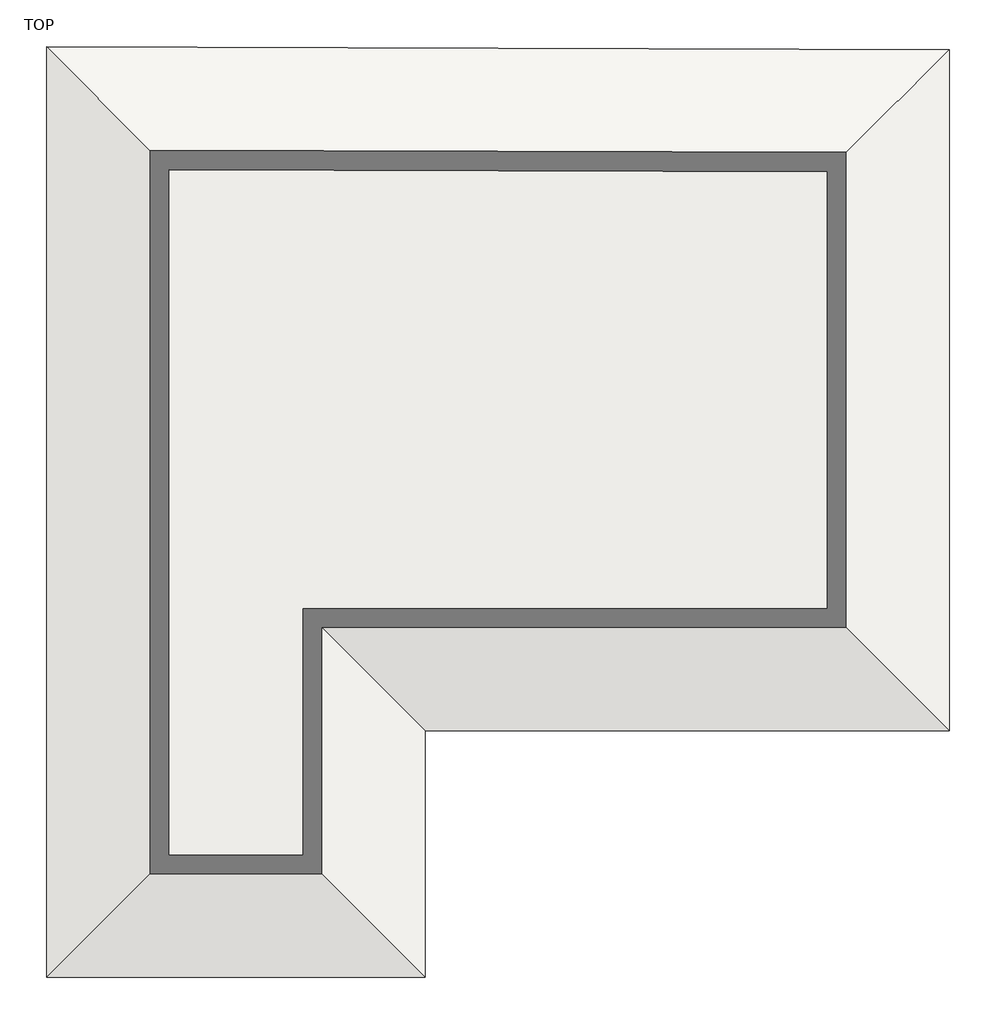
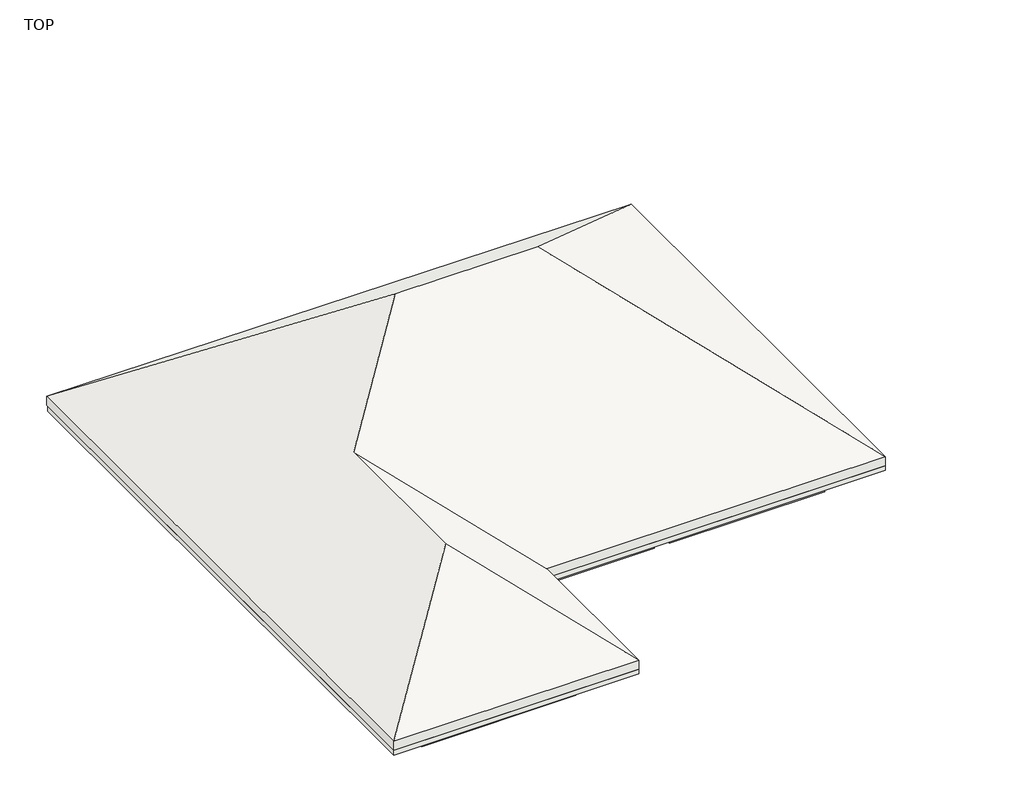
# One storey: 21 beams, 1 covering, 1 roof.
"""IFC4 building model written with IfcOpenShell, lengths in millimetres."""

from ifc_helpers import new_model, si_unit, frame, origin, place, context, project, spatial, polyline, outline, extrude, faceted_brep, element, save

model = new_model("IFC4")

# Units and contexts
model_context = context("Model", 3, world=origin())
ifc_project = project(units=[si_unit("LENGTHUNIT", "METRE", prefix="MILLI")], contexts=[model_context])

# Site, building, storey
site = spatial("IfcSite", under=ifc_project)
building = spatial("IfcBuilding", under=site)
storey = spatial("IfcBuildingStorey", under=building, Name="TOP", Elevation=6400.8)

# Beams
placement = place(None, origin())
element("IfcBeam", 1, ObjectType="Concrete-Rectangular Beam : 12 x 24", at=placement, inside=storey, context=model_context, shape_type="SweptSolid", body=[
    extrude(outline(polyline([(-11339.0293601, -6018.4747117), (-11643.8293601, -6018.4747117), (-11643.8293601, -2868.8747117), (-11339.0293601, -2868.8747117), (-11339.0293601, -6018.4747117)])), frame((0.0, 0.0, 5791.2), z_axis=(0.0, 0.0, 1.0), x_axis=(1.0, 0.0, 0.0)), (0.0, 0.0, 1.0), 609.6),
])
element("IfcBeam", 2, ObjectType="Concrete-Rectangular Beam : 12 x 24", at=placement, inside=storey, context=model_context, shape_type="SweptSolid", body=[
    extrude(outline(polyline([(-8251.5270642, -2564.0747117), (-8251.5270642, -2868.8747117), (-11339.0293601, -2868.8747117), (-11339.0293601, -2564.0747117), (-8251.5270642, -2564.0747117)])), frame((0.0, 0.0, 5791.2), z_axis=(0.0, 0.0, 1.0), x_axis=(1.0, 0.0, 0.0)), (0.0, 0.0, 1.0), 609.6),
])
element("IfcBeam", 3, ObjectType="Concrete-Rectangular Beam : 12 x 24", at=placement, inside=storey, context=model_context, shape_type="SweptSolid", body=[
    extrude(outline(polyline([(-4797.1270642, -2564.0747117), (-4797.1270642, -2868.8747117), (-7946.7270642, -2868.8747117), (-7946.7270642, -2564.0747117), (-4797.1270642, -2564.0747117)])), frame((0.0, 0.0, 5791.2), z_axis=(0.0, 0.0, 1.0), x_axis=(1.0, 0.0, 0.0)), (0.0, 0.0, 1.0), 609.6),
])
element("IfcBeam", 4, ObjectType="Concrete-Rectangular Beam : 12 x 24", at=placement, inside=storey, context=model_context, shape_type="SweptSolid", body=[
    extrude(outline(polyline([(-1351.9658472, -2564.0747117), (-1351.9658472, -2868.8747117), (-4492.3270642, -2868.8747117), (-4492.3270642, -2564.0747117), (-1351.9658472, -2564.0747117)])), frame((0.0, 0.0, 5791.2), z_axis=(0.0, 0.0, 1.0), x_axis=(1.0, 0.0, 0.0)), (0.0, 0.0, 1.0), 609.6),
])
element("IfcBeam", 5, ObjectType="Concrete-Rectangular Beam : 12 x 24", at=placement, inside=storey, context=model_context, shape_type="SweptSolid", body=[
    extrude(outline(polyline([(-1047.1658472, -5993.0747117), (-1351.9658472, -5993.0747117), (-1351.9658472, -2868.8747117), (-1047.1658472, -2868.8747117), (-1047.1658472, -5993.0747117)])), frame((0.0, 0.0, 5791.2), z_axis=(0.0, 0.0, 1.0), x_axis=(1.0, 0.0, 0.0)), (0.0, 0.0, 1.0), 609.6),
])
element("IfcBeam", 6, ObjectType="Concrete-Rectangular Beam : 12 x 24", at=placement, inside=storey, context=model_context, shape_type="SweptSolid", body=[
    extrude(outline(polyline([(-8251.5270642, -2868.8747117), (-7946.7270642, -2868.8747117), (-7946.7270642, -5993.0747117), (-8251.5270642, -5993.0747117), (-8251.5270642, -2868.8747117)])), frame((0.0, 0.0, 5791.2), z_axis=(0.0, 0.0, 1.0), x_axis=(1.0, 0.0, 0.0)), (0.0, 0.0, 1.0), 609.6),
    extrude(outline(polyline([(-7946.7270642, -6323.2747117), (-8251.5270642, -6323.2747117), (-8251.5270642, -6297.8747117), (-7946.7270642, -6297.8747117), (-7946.7270642, -6323.2747117)])), frame((0.0, 0.0, 5791.2), z_axis=(0.0, 0.0, 1.0), x_axis=(1.0, 0.0, 0.0)), (0.0, 0.0, 1.0), 609.6),
])
element("IfcBeam", 7, ObjectType="Concrete-Rectangular Beam : 12 x 24", at=placement, inside=storey, context=model_context, shape_type="SweptSolid", body=[
    extrude(outline(polyline([(-1047.1658472, -9984.0050402), (-1351.9658472, -9984.0050402), (-1351.9658472, -6297.8747117), (-1047.1658472, -6297.8747117), (-1047.1658472, -9984.0050402)])), frame((0.0, 0.0, 5791.2), z_axis=(0.0, 0.0, 1.0), x_axis=(1.0, 0.0, 0.0)), (0.0, 0.0, 1.0), 609.6),
])
element("IfcBeam", 8, ObjectType="Concrete-Rectangular Beam : 12 x 24", at=placement, inside=storey, context=model_context, shape_type="SweptSolid", body=[
    extrude(outline(polyline([(-4492.3270642, -10288.8050402), (-4492.3270642, -9984.0050402), (-1351.9658472, -9984.0050402), (-1351.9658472, -10288.8050402), (-4492.3270642, -10288.8050402)])), frame((0.0, 0.0, 5791.2), z_axis=(0.0, 0.0, 1.0), x_axis=(1.0, 0.0, 0.0)), (0.0, 0.0, 1.0), 609.6),
])
element("IfcBeam", 9, ObjectType="Concrete-Rectangular Beam : 12 x 24", at=placement, inside=storey, context=model_context, shape_type="Brep", body=[
    faceted_brep([(-7946.7270642, -9984.0050402, 6400.8), (-7946.7270642, -10288.8050402, 6400.8), (-7921.3270642, -10288.8050402, 6400.8), (-4797.1270642, -10288.8050402, 6400.8), (-4797.1270642, -9984.0050402, 6400.8), (-7946.7270642, -9984.0050402, 5791.2), (-4797.1270642, -9984.0050402, 5791.2), (-7946.7270642, -10288.8050402, 5791.2), (-4797.1270642, -10288.8050402, 5791.2), (-7921.3270642, -10288.8050402, 5791.2)], [[[0, 1, 2, 3, 4]], [[5, 0, 4, 6]], [[7, 5, 6, 8, 9]], [[1, 7, 9, 8, 3, 2]], [[1, 0, 5, 7]], [[3, 8, 6, 4]]]),
])
element("IfcBeam", 10, ObjectType="Concrete-Rectangular Beam : 12 x 24", at=placement, inside=storey, context=model_context, shape_type="SweptSolid", body=[
    extrude(outline(polyline([(-8251.5270642, -8902.7373391), (-7946.7270642, -8902.7373391), (-7946.7270642, -9984.0050402), (-8251.5270642, -9984.0050402), (-8251.5270642, -8902.7373391)])), frame((0.0, 0.0, 5791.2), z_axis=(0.0, 0.0, 1.0), x_axis=(1.0, 0.0, 0.0)), (0.0, 0.0, 1.0), 609.6),
])
element("IfcBeam", 11, ObjectType="Concrete-Rectangular Beam : 12 x 24", at=placement, inside=storey, context=model_context, shape_type="SweptSolid", body=[
    extrude(outline(polyline([(-7946.7270642, -8597.9373391), (-8251.5270642, -8597.9373391), (-8251.5270642, -6323.2747117), (-7946.7270642, -6323.2747117), (-7946.7270642, -8597.9373391)])), frame((0.0, 0.0, 5791.2), z_axis=(0.0, 0.0, 1.0), x_axis=(1.0, 0.0, 0.0)), (0.0, 0.0, 1.0), 609.6),
])
element("IfcBeam", 12, ObjectType="Concrete-Rectangular Beam : 12 x 24", at=placement, inside=storey, context=model_context, shape_type="SweptSolid", body=[
    extrude(outline(polyline([(-11339.0293601, -8902.7373391), (-11339.0293601, -8597.9373391), (-8251.5270642, -8597.9373391), (-8251.5270642, -8902.7373391), (-11339.0293601, -8902.7373391)])), frame((0.0, 0.0, 5791.2), z_axis=(0.0, 0.0, 1.0), x_axis=(1.0, 0.0, 0.0)), (0.0, 0.0, 1.0), 609.6),
])
element("IfcBeam", 13, ObjectType="Concrete-Rectangular Beam : 12 x 24", at=placement, inside=storey, context=model_context, shape_type="SweptSolid", body=[
    extrude(outline(polyline([(-11643.8293601, -6323.2747117), (-11339.0293601, -6323.2747117), (-11339.0293601, -8597.9373391), (-11643.8293601, -8597.9373391), (-11643.8293601, -6323.2747117)])), frame((0.0, 0.0, 5791.2), z_axis=(0.0, 0.0, 1.0), x_axis=(1.0, 0.0, 0.0)), (0.0, 0.0, 1.0), 609.6),
])
element("IfcBeam", 14, ObjectType="Concrete-Rectangular Beam : 12 x 24", at=placement, inside=storey, context=model_context, shape_type="Brep", body=[
    faceted_brep([(-8251.5270642, -6018.4747117, 6400.8), (-8251.5270642, -6297.8747117, 6400.8), (-8251.5270642, -6323.2747117, 6400.8), (-8251.5270642, -6323.2747117, 5791.2), (-8251.5270642, -6297.8747117, 5791.2), (-8251.5270642, -6018.4747117, 5791.2), (-11339.0293601, -6018.4747117, 6400.8), (-11339.0293601, -6323.2747117, 6400.8), (-11339.0293601, -6323.2747117, 5791.2), (-11339.0293601, -6018.4747117, 5791.2)], [[[0, 1, 2, 3, 4, 5]], [[2, 1, 0, 6, 7]], [[3, 2, 7, 8]], [[5, 4, 3, 8, 9]], [[0, 5, 9, 6]], [[6, 9, 8, 7]]]),
])
element("IfcBeam", 15, ObjectType="Concrete-Rectangular Beam : 12 x 24", at=placement, inside=storey, context=model_context, shape_type="SweptSolid", body=[
    extrude(outline(polyline([(-4797.1270642, -6297.8747117), (-4492.3270642, -6297.8747117), (-4492.3270642, -9984.0050402), (-4797.1270642, -9984.0050402), (-4797.1270642, -6297.8747117)])), frame((0.0, 0.0, 5791.2), z_axis=(0.0, 0.0, 1.0), x_axis=(1.0, 0.0, 0.0)), (0.0, 0.0, 1.0), 609.6),
])
element("IfcBeam", 16, ObjectType="Concrete-Rectangular Beam : 12 x 24", at=placement, inside=storey, context=model_context, shape_type="SweptSolid", body=[
    extrude(outline(polyline([(-4492.3270642, -6297.8747117), (-4492.3270642, -5993.0747117), (-1351.9658472, -5993.0747117), (-1351.9658472, -6297.8747117), (-4492.3270642, -6297.8747117)])), frame((0.0, 0.0, 5791.2), z_axis=(0.0, 0.0, 1.0), x_axis=(1.0, 0.0, 0.0)), (0.0, 0.0, 1.0), 609.6),
])
element("IfcBeam", 17, ObjectType="Concrete-Rectangular Beam : 12 x 24", at=placement, inside=storey, context=model_context, shape_type="SweptSolid", body=[
    extrude(outline(polyline([(-4797.1270642, -2868.8747117), (-4492.3270642, -2868.8747117), (-4492.3270642, -5993.0747117), (-4797.1270642, -5993.0747117), (-4797.1270642, -2868.8747117)])), frame((0.0, 0.0, 5791.2), z_axis=(0.0, 0.0, 1.0), x_axis=(1.0, 0.0, 0.0)), (0.0, 0.0, 1.0), 609.6),
])
element("IfcBeam", 18, ObjectType="Concrete-Rectangular Beam : 12 x 24", at=placement, inside=storey, context=model_context, shape_type="SweptSolid", body=[
    extrude(outline(polyline([(-4797.1270642, -5993.0747117), (-4797.1270642, -6297.8747117), (-7946.7270642, -6297.8747117), (-7946.7270642, -5993.0747117), (-4797.1270642, -5993.0747117)])), frame((0.0, 0.0, 5791.2), z_axis=(0.0, 0.0, 1.0), x_axis=(1.0, 0.0, 0.0)), (0.0, 0.0, 1.0), 609.6),
])
element("IfcBeam", 19, ObjectType="Concrete-Rectangular Beam : 12 x 24", at=placement, inside=storey, context=model_context, shape_type="SweptSolid", body=[
    extrude(outline(polyline([(-11643.8293601, -8902.7373391), (-11339.0293601, -8902.7373391), (-11339.0293601, -13183.002305), (-11643.8293601, -13183.002305), (-11643.8293601, -8902.7373391)])), frame((0.0, 0.0, 5791.2), z_axis=(0.0, 0.0, 1.0), x_axis=(1.0, 0.0, 0.0)), (0.0, 0.0, 1.0), 609.6),
])
element("IfcBeam", 20, ObjectType="Concrete-Rectangular Beam : 12 x 24", at=placement, inside=storey, context=model_context, shape_type="Brep", body=[
    faceted_brep([(-7921.3270642, -10288.8050402, 6400.8), (-7946.7270642, -10288.8050402, 6400.8), (-8226.1270642, -10288.8050402, 6400.8), (-8226.1270642, -13183.002305, 6400.8), (-7921.3270642, -13183.002305, 6400.8), (-8226.1270642, -10288.8050402, 5791.2), (-8226.1270642, -13183.002305, 5791.2), (-7946.7270642, -10288.8050402, 5791.2), (-7921.3270642, -10288.8050402, 5791.2), (-7921.3270642, -13183.002305, 5791.2)], [[[0, 1, 2, 3, 4]], [[2, 5, 6, 3]], [[5, 7, 8, 9, 6]], [[8, 0, 4, 9]], [[0, 8, 7, 5, 2, 1]], [[4, 3, 6, 9]]]),
])
element("IfcBeam", 21, ObjectType="Concrete-Rectangular Beam : 12 x 24", at=placement, inside=storey, context=model_context, shape_type="SweptSolid", body=[
    extrude(outline(polyline([(-11339.0293601, -13487.802305), (-11339.0293601, -13183.002305), (-8226.1270642, -13183.002305), (-8226.1270642, -13487.802305), (-11339.0293601, -13487.802305)])), frame((0.0, 0.0, 5791.2), z_axis=(0.0, 0.0, 1.0), x_axis=(1.0, 0.0, 0.0)), (0.0, 0.0, 1.0), 609.6),
])

# Covering
element("IfcCovering", 22, at=placement, inside=storey, context=model_context, shape_type="SweptSolid", body=[
    extrude(outline(polyline([(-12255.3236584, -14097.402305), (-12255.3236584, -1993.0926533), (-469.7236584, -1993.0926533), (-469.7236584, -10880.9896616), (-7311.7270642, -10880.9896616), (-7311.7270642, -14097.402305), (-12255.3236584, -14097.402305)])), frame((0.0, 0.0, 6299.2), z_axis=(0.0, 0.0, 1.0), x_axis=(1.0, 0.0, 0.0)), (0.0, 0.0, 1.0), 101.6),
])

# Roof
element("IfcRoof", 23, ObjectType="ROOFING 6\"", at=placement, inside=storey, context=model_context, shape_type="Brep", body=[
    faceted_brep([(-12255.3236584, -14097.402305, 6400.8), (-9783.5253613, -11625.6040078, 8254.6487228), (-7311.7270642, -14097.402305, 6400.8), (-7311.7270642, -10880.9896616, 6400.8), (-9783.5253613, -8409.1913644, 8254.6487228), (-7798.7248226, -6424.3908258, 9743.2491268), (-4921.3507509, -6429.3625691, 9739.5203194), (-469.7236584, -10880.9896616, 6400.8), (-469.7236584, -1993.0926533, 6400.8), (-12255.3236584, -1952.36444, 6400.8), (-12255.3236584, -14097.402305, 6591.3), (-7311.7270642, -14097.402305, 6591.3), (-9783.5253613, -11625.6040078, 8445.1487228), (-7311.7270642, -10880.9896616, 6591.3), (-9783.5253613, -8409.1913644, 8445.1487228), (-469.7236584, -10880.9896616, 6591.3), (-4921.3507509, -6429.3625691, 9930.0203194), (-7798.7248226, -6424.3908258, 9933.7491268), (-469.7236584, -1993.0926533, 6591.3), (-12255.3236584, -1952.36444, 6591.3)], [[[0, 1, 2]], [[3, 2, 1, 4]], [[3, 4, 5, 6, 7]], [[7, 6, 8]], [[1, 0, 9, 5, 4]], [[8, 6, 5, 9]], [[10, 11, 12]], [[11, 13, 14, 12]], [[13, 15, 16, 17, 14]], [[15, 18, 16]], [[10, 12, 14, 17, 19]], [[18, 19, 17, 16]], [[2, 11, 10, 0]], [[3, 13, 11, 2]], [[7, 15, 13, 3]], [[8, 18, 15, 7]], [[9, 19, 18, 8]], [[0, 10, 19, 9]]]),
])

save(model, "model.ifc")

# Revit data of these elements
# Type "Concrete-Rectangular Beam : 12 x 24"
#   Assembly Code = "B10"
#   Length [instance default] = 5' - 0"
#   b = 1' - 0"
#   h = 2' - 0"
#   Structural Material [instance default] = Concrete, Cast-in-Place gray
# Type
#   built-in parameter 1002203 = 1 (stored number, unit not read)
#   built-in parameter 1002202 = 1 (stored number, unit not read)
# Type "ROOFING 6\""
#   Assembly Code = "B1020"
#   Layers, outside or top first: 0' - 6" "ROOFING 6\"" (function 1)
# Elements 1, 2, 3, 4, 5, 7, 8, 9, 13, 19, 20, 21 (IfcBeam, "Concrete-Rectangular Beam : 12 x 24")
#   Structural Material = Concrete, Cast-in-Place gray
#   Phase Created = New Construction
#   Materials on its faces: "Concrete, Cast-in-Place gray", "beige colour"
# Elements 6, 10, 11, 12, 14, 15, 16, 17, 18 (IfcBeam, "Concrete-Rectangular Beam : 12 x 24")
#   Structural Material = Concrete, Cast-in-Place gray
#   Phase Created = New Construction
#   Materials on its faces: "Concrete, Cast-in-Place gray"
# Element 22 (IfcCovering)
#   Height Offset From Level = -0' - 4"
#   Phase Created = New Construction
# Element 23 (IfcRoof, "ROOFING 6\"")
#   built-in parameter 1001705 = 32.591 (stored number, unit not read)
#   built-in parameter 1001710 = 33615
#   Phase Created = New Construction
#   Materials on its faces: "ROOFING 6\"", "beige colour"
# Materials
#   "Concrete, Cast-in-Place gray": class "Concrete", colour RGB 192 192 192, transparency 0, Description = "Cast-in-place concrete", Cost = 0
#   "ROOFING 6\"": class "Generic", colour RGB 120 120 120, transparency 0, Cost = 0
#   "beige colour": class "Generic", colour RGB 120 120 120, transparency 0, Cost = 0
